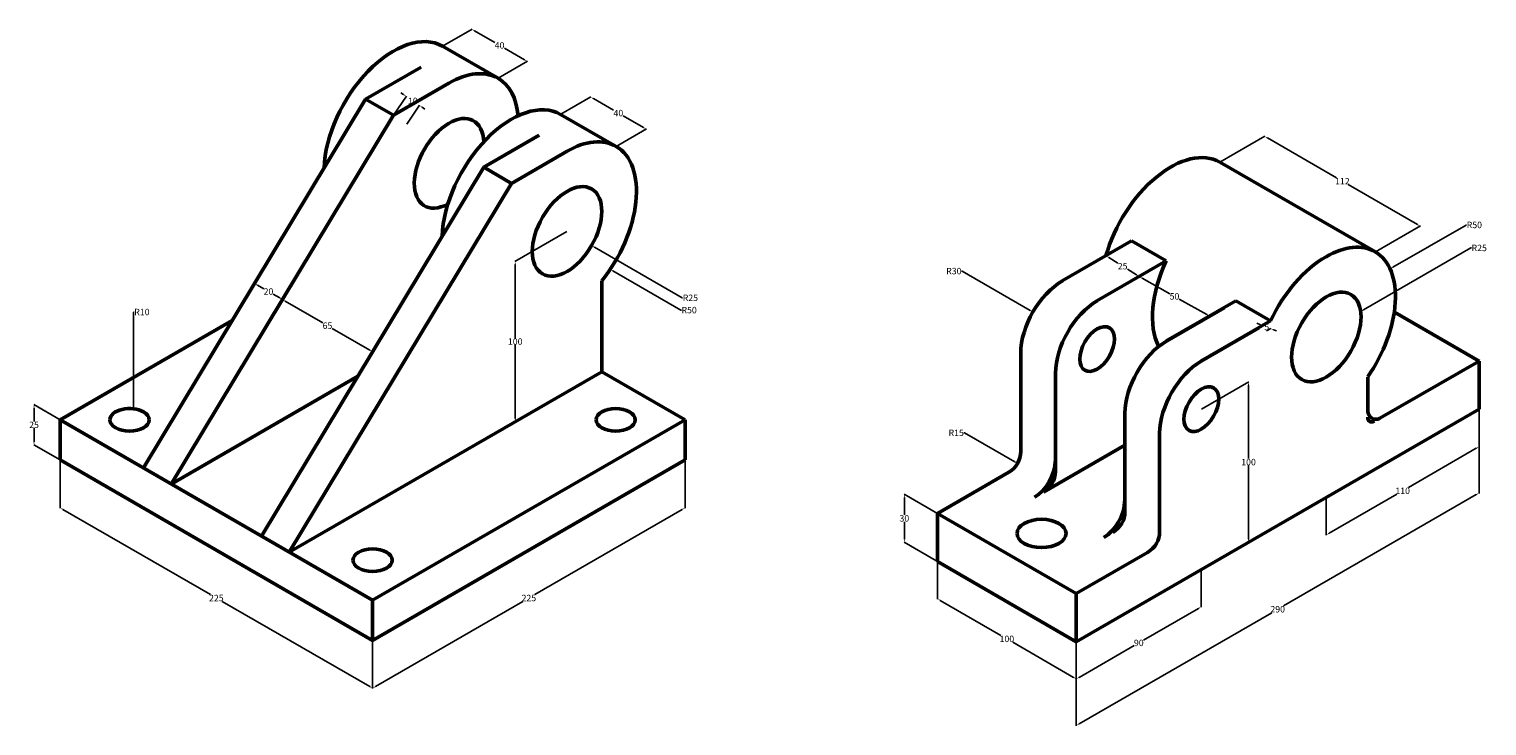
# Model space of a CAD drawing. Units: millimetres. Extents: x -183 to 726, y -48 to 387.
import ezdxf
from ezdxf import colors
from ezdxf.entities.mleader import LeaderData, LeaderLine
from ezdxf.math import Vec2, Vec3

# ---------------------------------------------------------------- set-up
doc = ezdxf.new("R2010")
doc.units = ezdxf.units.MM
doc.header["$MEASUREMENT"] = 0
for name, color, linetype, lineweight in [('M-DIMS', 2, 'Continuous', 25), ('M-OUTL', 7, 'Continuous', 50), ('M-TEXT', 3, 'Continuous', 25)]:
    doc.layers.add(name, color=color, linetype=linetype, lineweight=lineweight)
doc.styles.get("Standard").update_dxf_attribs({"font": 'arial.ttf'})
doc.dimstyles.get("Standard").update_dxf_attribs({"dimtxt": 4, "dimasz": 2, "dimexe": 0.18, "dimexo": 0.0625, "dimgap": 0.09, "dimtad": 0, "dimtih": 1, "dimtoh": 1, "dimdec": 0, "dimzin": 0, "dimdsep": 46, "dimtxsty": 'Standard', "dimcen": 0.09, "dimadec": 0, "dimazin": 0, "dimtfac": 1, "dimtdec": 0, "dimtofl": 0, "dimtmove": 0, "dimatfit": 3, "dimfxl": 1, "dimtolj": 1, "dimtzin": 0, "dimarcsym": 0})

# ---------------------------------------------------------------- blocks, each defined once
blk = doc.blocks.new('*D1')
at = {"layer": 'Defpoints', "color": 0, "transparency": 16777216}
for p in [(225.8, 118.04), (225.8, 88.2), (30.94, 5.54)]:
    blk.add_point(p, dxfattribs=at)
at = {"layer": 'M-DIMS', "color": 0, "lineweight": -2, "transparency": 16777216}
for p, q in [((225.8, 117.97), (225.8, 88)), ((224.07, 87.2), (132.06, 34.09)), ((32.67, -23.3), (124.68, 29.82)), ((30.94, 5.47), (30.94, -24.5))]:
    blk.add_line(p, q, dxfattribs=at)
at = {"layer": 'M-DIMS', "color": 0, "transparency": 16777216}
for points in [[(223.9, 87.49), (224.23, 86.91), (225.8, 88.2)], [(32.51, -23.01), (32.84, -23.59), (30.94, -24.3)]]:
    blk.add_solid(points, dxfattribs=at)
at = {"layer": 'M-DIMS', "color": 0, "transparency": 16777216, "insert": (128.37, 31.95), "char_height": 4, "attachment_point": 5}
blk.add_mtext('\\A1;225', dxfattribs=at)
blk = doc.blocks.new('*D2')
at = {"layer": 'Defpoints', "color": 0, "transparency": 16777216}
for p in [(-163.91, 118.04), (-163.91, 88.2), (30.94, 5.54)]:
    blk.add_point(p, dxfattribs=at)
at = {"layer": 'M-DIMS', "color": 0, "lineweight": -2, "transparency": 16777216}
for p, q in [((-163.91, 117.97), (-163.91, 88)), ((-162.18, 87.2), (-70.18, 34.09)), ((29.21, -23.3), (-62.79, 29.82)), ((30.94, 5.47), (30.94, -24.5))]:
    blk.add_line(p, q, dxfattribs=at)
at = {"layer": 'M-DIMS', "color": 0, "transparency": 16777216}
for points in [[(-162.01, 87.49), (-162.35, 86.91), (-163.91, 88.2)], [(29.38, -23.01), (29.04, -23.59), (30.94, -24.3)]]:
    blk.add_solid(points, dxfattribs=at)
at = {"layer": 'M-DIMS', "color": 0, "transparency": 16777216, "insert": (-66.49, 31.95), "char_height": 4, "attachment_point": 5}
blk.add_mtext('\\A1;225', dxfattribs=at)
blk = doc.blocks.new('*D3')
at = {"layer": 'Defpoints', "color": 0, "transparency": 16777216}
for p in [(-180.2, 152.44), (-163.91, 143.04), (-163.91, 118.04)]:
    blk.add_point(p, dxfattribs=at)
at = {"layer": 'M-DIMS', "color": 0, "lineweight": -2, "transparency": 16777216}
for p, q in [((-163.98, 143.08), (-180.38, 152.55)), ((-180.2, 150.44), (-180.2, 142.08)), ((-180.2, 129.44), (-180.2, 137.81)), ((-163.98, 118.08), (-180.38, 127.55))]:
    blk.add_line(p, q, dxfattribs=at)
at = {"layer": 'M-DIMS', "color": 0, "transparency": 16777216}
for points in [[(-180.53, 150.44), (-179.86, 150.44), (-180.2, 152.44)], [(-180.53, 129.44), (-179.86, 129.44), (-180.2, 127.44)]]:
    blk.add_solid(points, dxfattribs=at)
at = {"layer": 'M-DIMS', "color": 0, "transparency": 16777216, "insert": (-180.2, 139.94), "char_height": 4, "attachment_point": 5}
blk.add_mtext('\\A1;25', dxfattribs=at)
blk = doc.blocks.new('*D4')
at = {"layer": 'Defpoints', "color": 0, "transparency": 16777216}
for p in [(-25.35, 218.04), (30.94, 185.54), (30.94, 185.54)]:
    blk.add_point(p, dxfattribs=at)
at = {"layer": 'M-DIMS', "color": 0, "lineweight": -2, "transparency": 16777216}
for p, q in [((-25.32, 218.1), (-25.26, 218.2)), ((-23.62, 217.04), (-0.18, 203.51)), ((29.21, 186.54), (5.78, 200.07)), ((30.97, 185.6), (31.03, 185.7))]:
    blk.add_line(p, q, dxfattribs=at)
at = {"layer": 'M-DIMS', "color": 0, "transparency": 16777216}
for points in [[(-23.45, 217.33), (-23.78, 216.75), (-25.35, 218.04)], [(29.38, 186.83), (29.04, 186.25), (30.94, 185.54)]]:
    blk.add_solid(points, dxfattribs=at)
at = {"layer": 'M-DIMS', "color": 0, "transparency": 16777216, "insert": (2.8, 201.79), "char_height": 4, "attachment_point": 5}
blk.add_mtext('\\A1;65', dxfattribs=at)
blk = doc.blocks.new('*D5')
at = {"layer": 'Defpoints', "color": 0, "transparency": 16777216}
for p in [(-42.68, 228.02), (-42.67, 228.04), (-25.26, 218.2)]:
    blk.add_point(p, dxfattribs=at)
at = {"layer": 'M-DIMS', "color": 0, "lineweight": -2, "transparency": 16777216}
for p, q in [((-42.7, 227.99), (-42.77, 227.86)), ((-40.94, 227.04), (-36.96, 224.78)), ((-27.01, 219.16), (-31, 221.41)), ((-25.29, 218.14), (-25.36, 218.02))]:
    blk.add_line(p, q, dxfattribs=at)
at = {"layer": 'M-DIMS', "color": 0, "transparency": 16777216}
for points in [[(-40.78, 227.33), (-41.11, 226.75), (-42.68, 228.02)], [(-26.85, 219.45), (-27.18, 218.87), (-25.27, 218.18)]]:
    blk.add_solid(points, dxfattribs=at)
at = {"layer": 'M-DIMS', "color": 0, "transparency": 16777216, "insert": (-33.98, 223.1), "char_height": 4, "attachment_point": 5}
blk.add_mtext('\\A1;20', dxfattribs=at)
blk = doc.blocks.new('*D6')
at = {"layer": 'Defpoints', "color": 0, "transparency": 16777216}
for p in [(60.15, 339.13), (43.93, 333.04), (52.17, 327.42)]:
    blk.add_point(p, dxfattribs=at)
at = {"layer": 'M-DIMS', "color": 0, "lineweight": -2, "transparency": 16777216}
for p, q in [((50.27, 345.88), (48.61, 347)), ((43.97, 333.09), (52.02, 344.9)), ((52.2, 327.48), (60.26, 339.28)), ((61.81, 338), (63.46, 336.88))]:
    blk.add_line(p, q, dxfattribs=at)
at = {"layer": 'M-DIMS', "color": 0, "transparency": 16777216}
for points in [[(50.45, 346.15), (50.08, 345.6), (51.92, 344.75)], [(61.99, 338.28), (61.62, 337.73), (60.15, 339.13)]]:
    blk.add_solid(points, dxfattribs=at)
at = {"layer": 'M-DIMS', "color": 0, "transparency": 16777216, "insert": (56.04, 341.94), "char_height": 4, "attachment_point": 5}
blk.add_mtext('\\A1;10', dxfattribs=at)
blk = doc.blocks.new('*D7')
at = {"layer": 'Defpoints', "color": 0, "transparency": 16777216}
for p in [(74.55, 376.08), (127.43, 366.61), (109.19, 356.08)]:
    blk.add_point(p, dxfattribs=at)
at = {"layer": 'M-DIMS', "color": 0, "lineweight": -2, "transparency": 16777216}
for p, q in [((74.61, 376.11), (92.97, 386.71)), ((94.53, 385.61), (107.08, 378.36)), ((125.7, 367.61), (113.14, 374.86)), ((109.25, 356.11), (127.61, 366.71))]:
    blk.add_line(p, q, dxfattribs=at)
at = {"layer": 'M-DIMS', "color": 0, "transparency": 16777216}
for points in [[(94.69, 385.9), (94.36, 385.32), (92.79, 386.61)], [(125.87, 367.9), (125.54, 367.32), (127.43, 366.61)]]:
    blk.add_solid(points, dxfattribs=at)
at = {"layer": 'M-DIMS', "color": 0, "transparency": 16777216, "insert": (110.11, 376.61), "char_height": 4, "attachment_point": 5}
blk.add_mtext('\\A1;40', dxfattribs=at)
blk = doc.blocks.new('*D8')
at = {"layer": 'Defpoints', "color": 0, "transparency": 16777216}
for p in [(148.16, 333.58), (201.51, 324.38), (182.8, 313.58)]:
    blk.add_point(p, dxfattribs=at)
at = {"layer": 'M-DIMS', "color": 0, "lineweight": -2, "transparency": 16777216}
for p, q in [((148.23, 333.61), (167.05, 344.48)), ((168.6, 343.38), (181.16, 336.12)), ((199.78, 325.38), (187.22, 332.63)), ((182.87, 313.61), (201.69, 324.48))]:
    blk.add_line(p, q, dxfattribs=at)
at = {"layer": 'M-DIMS', "color": 0, "transparency": 16777216}
for points in [[(168.77, 343.66), (168.43, 343.09), (166.87, 344.38)], [(199.95, 325.66), (199.61, 325.09), (201.51, 324.38)]]:
    blk.add_solid(points, dxfattribs=at)
at = {"layer": 'M-DIMS', "color": 0, "transparency": 16777216, "insert": (184.19, 334.38), "char_height": 4, "attachment_point": 5}
blk.add_mtext('\\A1;40', dxfattribs=at)
blk = doc.blocks.new('*D9')
at = {"layer": 'Defpoints', "color": 0, "transparency": 16777216}
for p in [(152.19, 260.54), (152.19, 160.54), (119.86, 141.88)]:
    blk.add_point(p, dxfattribs=at)
at = {"layer": 'M-DIMS', "color": 0, "lineweight": -2, "transparency": 16777216}
for p, q in [((152.12, 260.51), (119.68, 241.78)), ((119.86, 239.88), (119.86, 194.01)), ((119.86, 143.88), (119.86, 189.75)), ((152.12, 160.51), (119.68, 141.78))]:
    blk.add_line(p, q, dxfattribs=at)
at = {"layer": 'M-DIMS', "color": 0, "transparency": 16777216}
for points in [[(119.53, 239.88), (120.2, 239.88), (119.86, 241.88)], [(119.53, 143.88), (120.2, 143.88), (119.86, 141.88)]]:
    blk.add_solid(points, dxfattribs=at)
at = {"layer": 'M-DIMS', "color": 0, "transparency": 16777216, "insert": (119.86, 191.88), "char_height": 4, "attachment_point": 5}
blk.add_mtext('\\A1;100', dxfattribs=at)
blk = doc.blocks.new('*D10')
at = {"layer": 'Defpoints', "color": 0, "transparency": 16777216}
for p in [(720.9, 149.72), (720.9, 97.43), (469.75, 4.72)]:
    blk.add_point(p, dxfattribs=at)
at = {"layer": 'M-DIMS', "color": 0, "lineweight": -2, "transparency": 16777216}
for p, q in [((720.9, 149.64), (720.9, 97.22)), ((719.17, 96.43), (599.02, 27.06)), ((471.49, -46.57), (591.64, 22.8)), ((469.75, 4.64), (469.75, -47.78))]:
    blk.add_line(p, q, dxfattribs=at)
at = {"layer": 'M-DIMS', "color": 0, "transparency": 16777216}
for points in [[(719, 96.72), (719.34, 96.14), (720.9, 97.43)], [(471.32, -46.28), (471.65, -46.86), (469.75, -47.57)]]:
    blk.add_solid(points, dxfattribs=at)
at = {"layer": 'M-DIMS', "color": 0, "transparency": 16777216, "insert": (595.33, 24.93), "char_height": 4, "attachment_point": 5}
blk.add_mtext('\\A1;290', dxfattribs=at)
blk = doc.blocks.new('*D11')
at = {"layer": 'Defpoints', "color": 0, "transparency": 16777216}
for p in [(547.7, 49.72), (547.7, 26.46), (469.75, 4.72)]:
    blk.add_point(p, dxfattribs=at)
at = {"layer": 'M-DIMS', "color": 0, "lineweight": -2, "transparency": 16777216}
for p, q in [((547.7, 49.64), (547.7, 26.26)), ((545.97, 25.46), (511.67, 5.67)), ((469.75, 4.64), (469.75, -18.74)), ((471.49, -17.54), (505.78, 2.26))]:
    blk.add_line(p, q, dxfattribs=at)
at = {"layer": 'M-DIMS', "color": 0, "transparency": 16777216}
for points in [[(545.8, 25.75), (546.13, 25.17), (547.7, 26.46)], [(471.32, -17.25), (471.65, -17.83), (469.75, -18.54)]]:
    blk.add_solid(points, dxfattribs=at)
at = {"layer": 'M-DIMS', "color": 0, "transparency": 16777216, "insert": (508.73, 3.96), "char_height": 4, "attachment_point": 5}
blk.add_mtext('\\A1;90', dxfattribs=at)
blk = doc.blocks.new('*D12')
at = {"layer": 'Defpoints', "color": 0, "transparency": 16777216}
for p in [(720.9, 149.72), (720.9, 126.33), (625.64, 94.72)]:
    blk.add_point(p, dxfattribs=at)
at = {"layer": 'M-DIMS', "color": 0, "lineweight": -2, "transparency": 16777216}
for p, q in [((720.9, 149.64), (720.9, 126.13)), ((719.17, 125.33), (676.96, 100.97)), ((625.64, 94.64), (625.64, 71.13)), ((627.37, 72.33), (669.58, 96.7))]:
    blk.add_line(p, q, dxfattribs=at)
at = {"layer": 'M-DIMS', "color": 0, "transparency": 16777216}
for points in [[(719, 125.62), (719.34, 125.04), (720.9, 126.33)], [(627.2, 72.62), (627.54, 72.04), (625.64, 71.33)]]:
    blk.add_solid(points, dxfattribs=at)
at = {"layer": 'M-DIMS', "color": 0, "transparency": 16777216, "insert": (673.27, 98.83), "char_height": 4, "attachment_point": 5}
blk.add_mtext('\\A1;110', dxfattribs=at)
blk = doc.blocks.new('*D13')
at = {"layer": 'Defpoints', "color": 0, "transparency": 16777216}
for p in [(383.15, 54.72), (383.15, 31.46), (469.75, 4.72)]:
    blk.add_point(p, dxfattribs=at)
at = {"layer": 'M-DIMS', "color": 0, "lineweight": -2, "transparency": 16777216}
for p, q in [((383.15, 54.64), (383.15, 31.26)), ((384.88, 30.46), (422.76, 8.6)), ((468.02, -17.54), (430.15, 4.33)), ((469.75, 4.64), (469.75, -18.74))]:
    blk.add_line(p, q, dxfattribs=at)
at = {"layer": 'M-DIMS', "color": 0, "transparency": 16777216}
for points in [[(385.05, 30.75), (384.72, 30.17), (383.15, 31.46)], [(468.19, -17.25), (467.86, -17.83), (469.75, -18.54)]]:
    blk.add_solid(points, dxfattribs=at)
at = {"layer": 'M-DIMS', "color": 0, "transparency": 16777216, "insert": (426.45, 6.46), "char_height": 4, "attachment_point": 5}
blk.add_mtext('\\A1;100', dxfattribs=at)
blk = doc.blocks.new('*D14')
at = {"layer": 'Defpoints', "color": 0, "transparency": 16777216}
for p in [(383.15, 84.72), (362.52, 66.63), (383.15, 54.72)]:
    blk.add_point(p, dxfattribs=at)
at = {"layer": 'M-DIMS', "color": 0, "lineweight": -2, "transparency": 16777216}
for p, q in [((383.09, 84.75), (362.34, 96.73)), ((362.52, 94.63), (362.52, 83.76)), ((362.52, 68.63), (362.52, 79.5)), ((383.09, 54.75), (362.34, 66.73))]:
    blk.add_line(p, q, dxfattribs=at)
at = {"layer": 'M-DIMS', "color": 0, "transparency": 16777216}
for points in [[(362.18, 94.63), (362.85, 94.63), (362.52, 96.63)], [(362.18, 68.63), (362.85, 68.63), (362.52, 66.63)]]:
    blk.add_solid(points, dxfattribs=at)
at = {"layer": 'M-DIMS', "color": 0, "transparency": 16777216, "insert": (362.52, 81.63), "char_height": 4, "attachment_point": 5}
blk.add_mtext('\\A1;30', dxfattribs=at)
blk = doc.blocks.new('*D15')
at = {"layer": 'Defpoints', "color": 0, "transparency": 16777216}
for p in [(488.25, 245.39), (509.02, 232.39), (509.02, 232.39)]:
    blk.add_point(p, dxfattribs=at)
at = {"layer": 'M-DIMS', "color": 0, "lineweight": -2, "transparency": 16777216}
for p, q in [((488.31, 245.43), (488.42, 245.49)), ((489.94, 244.33), (495.63, 240.77)), ((507.33, 233.45), (501.64, 237.01)), ((509.08, 232.42), (509.2, 232.49))]:
    blk.add_line(p, q, dxfattribs=at)
at = {"layer": 'M-DIMS', "color": 0, "transparency": 16777216}
for points in [[(490.12, 244.61), (489.76, 244.05), (488.25, 245.39)], [(507.5, 233.73), (507.15, 233.16), (509.02, 232.39)]]:
    blk.add_solid(points, dxfattribs=at)
at = {"layer": 'M-DIMS', "color": 0, "transparency": 16777216, "insert": (498.63, 238.89), "char_height": 4, "attachment_point": 5}
blk.add_mtext('\\A1;25', dxfattribs=at)
blk = doc.blocks.new('*D16')
at = {"layer": 'Defpoints', "color": 0, "transparency": 16777216}
for p in [(509.02, 232.39), (552.94, 207.74), (552.94, 207.74)]:
    blk.add_point(p, dxfattribs=at)
at = {"layer": 'M-DIMS', "color": 0, "lineweight": -2, "transparency": 16777216}
for p, q in [((509.08, 232.42), (509.2, 232.49)), ((510.77, 231.41), (528.03, 221.72)), ((551.2, 208.72), (533.93, 218.41)), ((553.01, 207.78), (553.13, 207.85))]:
    blk.add_line(p, q, dxfattribs=at)
at = {"layer": 'M-DIMS', "color": 0, "transparency": 16777216}
for points in [[(510.93, 231.7), (510.6, 231.12), (509.02, 232.39)], [(551.36, 209.01), (551.04, 208.43), (552.94, 207.74)]]:
    blk.add_solid(points, dxfattribs=at)
at = {"layer": 'M-DIMS', "color": 0, "transparency": 16777216, "insert": (530.98, 220.07), "char_height": 4, "attachment_point": 5}
blk.add_mtext('\\A1;50', dxfattribs=at)
blk = doc.blocks.new('*D17')
at = {"layer": 'Defpoints', "color": 0, "transparency": 16777216}
for p in [(583.51, 200.39), (590.9, 200), (588.31, 198.5)]:
    blk.add_point(p, dxfattribs=at)
at = {"layer": 'M-DIMS', "color": 0, "lineweight": -2, "transparency": 16777216}
for p, q in [((584.23, 202.62), (582.37, 203.35)), ((583.57, 200.43), (586.3, 202)), ((588.38, 198.54), (591.1, 200.11)), ((592.76, 199.26), (594.62, 198.53))]:
    blk.add_line(p, q, dxfattribs=at)
at = {"layer": 'M-DIMS', "color": 0, "transparency": 16777216}
for points in [[(584.36, 202.93), (584.11, 202.31), (586.1, 201.89)], [(592.88, 199.57), (592.64, 198.95), (590.9, 200)]]:
    blk.add_solid(points, dxfattribs=at)
at = {"layer": 'M-DIMS', "color": 0, "transparency": 16777216, "insert": (588.5, 200.94), "char_height": 4, "attachment_point": 5}
blk.add_mtext('\\A1;5', dxfattribs=at)
blk = doc.blocks.new('*D18')
at = {"layer": 'Defpoints', "color": 0, "transparency": 16777216}
for p in [(587.16, 319.86), (559.26, 303.75), (656.26, 247.75)]:
    blk.add_point(p, dxfattribs=at)
at = {"layer": 'M-DIMS', "color": 0, "lineweight": -2, "transparency": 16777216}
for p, q in [((559.33, 303.78), (587.34, 319.96)), ((588.89, 318.86), (632.02, 293.95)), ((682.42, 264.86), (639.29, 289.76)), ((656.32, 247.78), (684.34, 263.96))]:
    blk.add_line(p, q, dxfattribs=at)
at = {"layer": 'M-DIMS', "color": 0, "transparency": 16777216}
for points in [[(589.06, 319.14), (588.73, 318.57), (587.16, 319.86)], [(682.59, 265.14), (682.26, 264.57), (684.16, 263.86)]]:
    blk.add_solid(points, dxfattribs=at)
at = {"layer": 'M-DIMS', "color": 0, "transparency": 16777216, "insert": (635.66, 291.86), "char_height": 4, "attachment_point": 5}
blk.add_mtext('\\A1;112', dxfattribs=at)
blk = doc.blocks.new('*D19')
at = {"layer": 'Defpoints', "color": 0, "transparency": 16777216}
for p in [(547.7, 149.72), (577.14, 66.71), (547.7, 49.72)]:
    blk.add_point(p, dxfattribs=at)
at = {"layer": 'M-DIMS', "color": 0, "lineweight": -2, "transparency": 16777216}
for p, q in [((547.76, 149.75), (577.32, 166.82)), ((577.14, 164.71), (577.14, 118.85)), ((577.14, 68.71), (577.14, 114.58)), ((547.76, 49.75), (577.32, 66.82))]:
    blk.add_line(p, q, dxfattribs=at)
at = {"layer": 'M-DIMS', "color": 0, "transparency": 16777216}
for points in [[(576.81, 164.71), (577.47, 164.71), (577.14, 166.71)], [(576.81, 68.71), (577.47, 68.71), (577.14, 66.71)]]:
    blk.add_solid(points, dxfattribs=at)
at = {"layer": 'M-DIMS', "color": 0, "transparency": 16777216, "insert": (577.14, 116.71), "char_height": 4, "attachment_point": 5}
blk.add_mtext('\\A1;100', dxfattribs=at)

msp = doc.modelspace()

# ---------------------------------------------------------------- linework, layer by layer
at = {"layer": 'M-OUTL'}
for p, q in [((109.19, 356.08), (74.55, 376.08)), ((61.25, 363.04), (26.61, 343.04)), ((78.57, 353.04), (43.93, 333.04)), ((26.61, 343.04), (-111.95, 113.04)), ((43.93, 333.04), (26.61, 343.04)), ((43.93, 333.04), (-94.63, 103.04)), ((148.16, 333.58), (182.8, 313.58)), ((134.87, 320.54), (100.22, 300.54)), ((152.19, 310.54), (117.54, 290.54)), ((100.22, 300.54), (-38.34, 70.54)), ((117.54, 290.54), (100.22, 300.54)), ((559.26, 303.75), (656.26, 247.75)), ((117.54, 290.54), (-21.02, 60.54)), ((460.92, 229.79), (504.23, 254.79)), ((525.88, 242.29), (504.23, 254.79)), ((482.57, 217.29), (525.88, 242.29)), ((173.84, 173.04), (173.84, 229.74)), ((525.88, 192.29), (569.18, 217.29)), ((526.05, 192.22), (561.86, 212.89)), ((590.83, 204.79), (569.18, 217.29)), ((720.9, 179.72), (668.21, 210.14)), ((-163.91, 143.04), (-56.53, 205.04)), ((547.53, 179.79), (590.83, 204.79)), ((547.7, 179.72), (583.51, 200.39)), ((435.11, 184.72), (435.11, 123.38)), ((173.84, 173.04), (-21.02, 60.54)), ((225.8, 143.04), (173.84, 173.04)), ((720.9, 179.72), (659.12, 144.05)), ((720.9, 149.72), (720.9, 179.72)), ((-94.63, 103.04), (21.7, 170.21)), ((456.76, 172.22), (456.76, 110.88)), ((651.62, 148.38), (651.62, 169.72)), ((469.75, 4.72), (720.9, 149.72)), ((500.07, 147.22), (500.07, 85.88)), ((30.94, 30.54), (-163.91, 143.04)), ((-163.91, 143.04), (-163.91, 118.04)), ((30.94, 30.54), (225.8, 143.04)), ((225.8, 143.04), (225.8, 118.04)), ((521.72, 134.72), (521.72, 73.38)), ((449.26, 97.89), (500.07, 127.22)), ((-163.91, 118.04), (30.94, 5.54)), ((225.8, 118.04), (30.94, 5.54)), ((383.15, 84.72), (427.61, 110.39)), ((383.15, 54.72), (383.15, 84.72)), ((383.15, 84.72), (469.75, 34.72)), ((469.75, 4.72), (383.15, 54.72)), ((514.22, 60.39), (469.75, 34.72)), ((30.94, 5.54), (30.94, 30.54)), ((469.75, 34.72), (469.75, 4.72))]:
    msp.add_line(p, q, dxfattribs=at)
for centre, radius, start, end in [((656.62, 148.38), 5, 180, 300), ((420.11, 123.38), 15, 300, 360), ((441.76, 110.88), 15, 300, 360), ((485.07, 85.88), 15, 300, 360), ((506.72, 73.38), 15, 300, 360)]:
    msp.add_arc(centre, radius, start, end, dxfattribs=at)
for centre, major_axis, start_param, end_param in [((43.93, 323.04), (-30.62, -53.03), 3.141593, 5.459594), ((78.57, 303.04), (30.62, 53.03), 0, 0.785398), ((78.57, 303.04), (30.62, 53.03), 5.593368, 6.283185), ((117.54, 280.54), (-30.62, -53.03), 3.141593, 5.459594), ((78.57, 303.04), (-15.31, -26.52), 2.388996, 7.035782), ((152.19, 260.54), (30.62, 53.03), 0, 0.785398), ((152.19, 260.54), (30.62, 53.03), 4.45059, 6.283185), ((528.64, 250.72), (-30.62, -53.03), 9.424778, 11.412705), ((625.47, 194.79), (30.62, 53.03), 0, 0.785398), ((625.47, 194.79), (30.62, 53.03), 4.570492, 6.283185), ((560.52, 232.29), (30.62, 53.03), 1.712693, 2.779217), ((625.47, 194.79), (30.62, 53.03), 0.785398, 1.712693), ((461.09, 199.72), (-18.37, -31.82), 3.926991, 5.497787), ((482.75, 187.22), (-18.37, -31.82), 3.926991, 5.497787), ((526.05, 162.22), (-18.37, -31.82), 3.926991, 5.497787), ((547.7, 149.72), (-18.37, -31.82), 3.926991, 5.497787), ((-120.61, 143.04), (12.25, 0), 0.785398, 3.141593), ((-120.61, 143.04), (12.25, 0), 0, 0.785398), ((-120.61, 143.04), (12.25, 0), 3.141593, 6.283185), ((655.78, 147.29), (-3.06, -5.3), 5.497787, 6.283185), ((655.78, 147.29), (-3.06, -5.3), 0, 0.785398), ((443.6, 109.79), (-9.19, -15.91), 0.785398, 2.356194), ((486.9, 84.79), (-9.19, -15.91), 0.785398, 2.356194)]:
    msp.add_ellipse(centre, major_axis=major_axis, ratio=0.57735, start_param=start_param, end_param=end_param, dxfattribs=at)
for centre, major_axis in [((152.19, 260.54), (-15.31, -26.52)), ((625.64, 194.72), (-15.31, -26.52)), ((482.75, 187.22), (-7.65, -13.26)), ((547.7, 149.72), (-7.65, -13.26)), ((182.5, 143.04), (-12.25, 0)), ((448.1, 72.22), (-15.31, 0)), ((30.94, 55.54), (-12.25, 0))]:
    msp.add_ellipse(centre, major_axis=major_axis, ratio=0.57735, dxfattribs=at)

# ---------------------------------------------------------------- dimensions: what is measured, and where the dimension line sits
at = {"layer": 'M-DIMS'}
for p1, p2, distance, picture, middle in [((74.55, 376.08), (109.19, 356.08), 18.24, '*D7', (110.11, 376.61)), ((43.93, 333.04), (52.17, 327.42), 14.17, '*D6', (56.04, 341.94)), ((148.16, 333.58), (182.8, 313.58), 18.71, '*D8', (184.19, 334.38)), ((656.26, 247.75), (559.26, 303.75), -27.9, '*D18', (635.66, 291.86)), ((152.19, 260.54), (152.19, 160.54), -32.32, '*D9', (119.86, 191.88)), ((488.25, 245.39), (509.02, 232.39), 0, '*D15', (498.63, 238.89)), ((-25.26, 218.2), (-42.67, 228.04), 0.03, '*D5', (-33.98, 223.1)), ((509.02, 232.39), (552.94, 207.74), 0, '*D16', (530.98, 220.07)), ((-25.35, 218.04), (30.94, 185.54), 0, '*D4', (2.8, 201.79)), ((583.51, 200.39), (588.31, 198.5), 2.34, '*D17', (588.5, 200.94)), ((547.7, 149.72), (547.7, 49.72), 29.44, '*D19', (577.14, 116.71)), ((-163.91, 118.04), (-163.91, 143.04), 16.28, '*D3', (-180.2, 139.94)), ((469.75, 4.72), (720.9, 149.72), -45.28, '*D10', (595.33, 24.93)), ((625.64, 94.72), (720.9, 149.72), -20.25, '*D12', (673.27, 98.83)), ((30.94, 5.54), (-163.91, 118.04), 25.84, '*D2', (-66.49, 31.95)), ((30.94, 5.54), (225.8, 118.04), -25.84, '*D1', (128.37, 31.95)), ((383.15, 84.72), (383.15, 54.72), -20.64, '*D14', (362.52, 81.63)), ((469.75, 4.72), (383.15, 54.72), 20.14, '*D13', (426.45, 6.46)), ((469.75, 4.72), (547.7, 49.72), -20.14, '*D11', (508.73, 3.96))]:
    dim = msp.add_aligned_dim(p1=p1, p2=p2, distance=distance, dimstyle='Standard', override={"dimclrd": 0, "dimclre": 0, "dimclrt": 0}, dxfattribs=at)
    dim.commit()
    dim.dimension.update_dxf_attribs({"geometry": picture, "text_midpoint": middle})

# ---------------------------------------------------------------- leaders
at = {"layer": 'M-TEXT'}
ml = msp.add_multileader_mtext('Standard', dxfattribs=at)
ml.set_content('R50', color=256)
ml.set_leader_properties()
ml.build(insert=Vec2(0, 0))
ml.multileader.update_dxf_attribs({"dogleg_length": 0.36, "arrow_head_size": 2})
ctx = ml.context
ctx.base_point, ctx.arrow_head_size, ctx.landing_gap_size, ctx.plane_origin = Vec3(713.12, 264.56), 2, 0.09, Vec3(665.49, 237.27)
notes = []
notes.append((ctx, [(0, (1, 1, 0), (712.76, 264.56), (1, 0), 0.36, [(0, [(665.49, 237.27)], 0, [])])]))
ctx.mtext.insert, ctx.mtext.flow_direction = Vec3(713.21, 266.6), 5
ml = msp.add_multileader_mtext('Standard', dxfattribs=at)
ml.set_content('R25', color=256)
ml.set_leader_properties()
ml.build(insert=Vec2(0, 0))
ml.multileader.update_dxf_attribs({"dogleg_length": 0.36, "arrow_head_size": 2})
ctx = ml.context
ctx.base_point, ctx.arrow_head_size, ctx.landing_gap_size, ctx.plane_origin = Vec3(224.25, 219.14), 2, 0.09, Vec3(167.5, 251.7)
notes.append((ctx, [(0, (1, 1, 0), (223.89, 219.14), (1, 0), 0.36, [(0, [(167.5, 251.7)], 0, [])])]))
ctx.mtext.insert, ctx.mtext.flow_direction = Vec3(224.34, 221.18), 5
ml = msp.add_multileader_mtext('Standard', dxfattribs=at)
ml.set_content('R25', color=256)
ml.set_leader_properties()
ml.build(insert=Vec2(0, 0))
ml.multileader.update_dxf_attribs({"dogleg_length": 0.36, "arrow_head_size": 2})
ctx = ml.context
ctx.base_point, ctx.arrow_head_size, ctx.landing_gap_size, ctx.plane_origin = Vec3(716.14, 250.23), 2, 0.09, Vec3(647.08, 210.57)
notes.append((ctx, [(0, (1, 1, 0), (715.78, 250.23), (1, 0), 0.36, [(0, [(647.08, 210.57)], 0, [])])]))
ctx.mtext.insert, ctx.mtext.flow_direction = Vec3(716.23, 252.26), 5
ml = msp.add_multileader_mtext('Standard', dxfattribs=at)
ml.set_content('R50', color=256)
ml.set_leader_properties()
ml.build(insert=Vec2(0, 0))
ml.multileader.update_dxf_attribs({"dogleg_length": 0.36, "arrow_head_size": 2})
ctx = ml.context
ctx.base_point, ctx.arrow_head_size, ctx.landing_gap_size, ctx.plane_origin = Vec3(223.46, 211.48), 2, 0.09, Vec3(179.08, 236.89)
notes.append((ctx, [(0, (1, 1, 0), (223.1, 211.48), (1, 0), 0.36, [(0, [(179.08, 236.89)], 0, [])])]))
ctx.mtext.insert, ctx.mtext.flow_direction = Vec3(223.55, 213.51), 5
ml = msp.add_multileader_mtext('Standard', dxfattribs=at)
ml.set_content('R30', color=256)
ml.set_leader_properties()
ml.build(insert=Vec2(0, 0))
ml.multileader.update_dxf_attribs({"dogleg_length": 0.36, "arrow_head_size": 2})
ctx = ml.context
ctx.base_point, ctx.arrow_head_size, ctx.landing_gap_size, ctx.plane_origin = Vec3(388.51, 235.8), 2, 0.09, Vec3(442.72, 210.32)
ctx.text_align_type = 2
notes.append((ctx, [(0, (1, 1, 0), (398.59, 235.8), (-1, 0), 0.36, [(0, [(442.72, 210.32)], 0, [])])]))
ctx.mtext.insert, ctx.mtext.alignment, ctx.mtext.flow_direction = Vec3(398.14, 237.84), 3, 5
ml = msp.add_multileader_mtext('Standard', dxfattribs=at)
ml.set_content('R10', color=256)
ml.set_leader_properties()
ml.build(insert=Vec2(0, 0))
ml.multileader.update_dxf_attribs({"dogleg_length": 0.36, "arrow_head_size": 2})
ctx = ml.context
ctx.base_point, ctx.arrow_head_size, ctx.landing_gap_size, ctx.plane_origin = Vec3(-117.77, 210.28), 2, 0.09, Vec3(-118.13, 148.68)
notes.append((ctx, [(0, (1, 1, 0), (-118.13, 210.28), (1, 0), 0.36, [(0, [(-118.13, 148.68)], 0, [])])]))
ctx.mtext.insert, ctx.mtext.flow_direction = Vec3(-117.68, 212.31), 5
ml = msp.add_multileader_mtext('Standard', dxfattribs=at)
ml.set_content('R15', color=256)
ml.set_leader_properties()
ml.build(insert=Vec2(0, 0))
ml.multileader.update_dxf_attribs({"dogleg_length": 0.36, "arrow_head_size": 2})
ctx = ml.context
ctx.base_point, ctx.arrow_head_size, ctx.landing_gap_size, ctx.plane_origin = Vec3(389.93, 134.96), 2, 0.09, Vec3(433.1, 115.88)
ctx.text_align_type = 2
notes.append((ctx, [(0, (1, 1, 0), (400.05, 134.96), (-1, 0), 0.36, [(0, [(433.1, 115.88)], 0, [])])]))
ctx.mtext.insert, ctx.mtext.alignment, ctx.mtext.flow_direction = Vec3(399.6, 136.99), 3, 5
for ctx, leaders in notes:
    for number, flags, end, landing, length, lines in leaders:
        leader = LeaderData()
        leader.index, (leader.has_last_leader_line, leader.has_dogleg_vector, leader.attachment_direction) = number, flags
        leader.last_leader_point, leader.dogleg_vector, leader.dogleg_length = Vec3(end), Vec3(landing), length
        for number, points, colour, breaks in lines:
            line = LeaderLine()
            line.index, line.vertices, line.color, line.breaks = number, Vec3.list(points), colors.encode_raw_color(colour), breaks
            leader.lines.append(line)
        ctx.leaders.append(leader)

doc.saveas('drawing.dxf')
